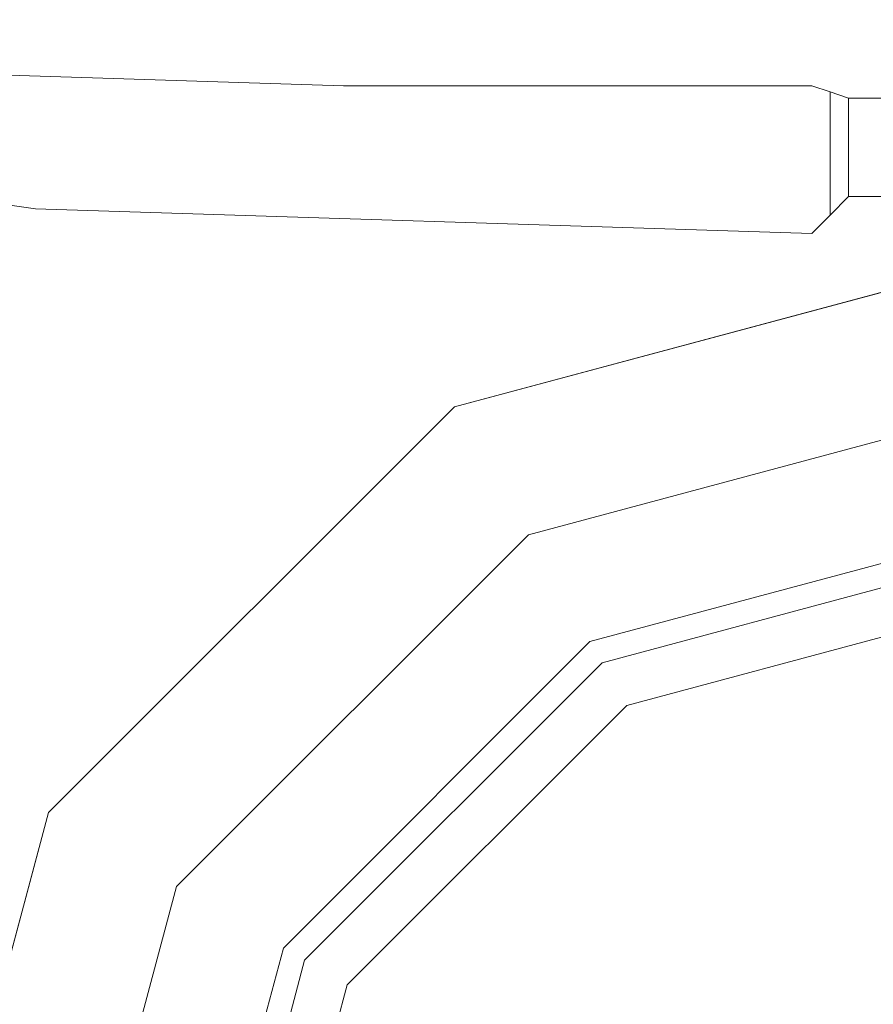
# Model space of a CAD drawing. Units: inches. Extents: x 375 to 1122, y 27 to 1069.
# Tile 144 of 155: x 734.829 to 739.094, y 896.928 to 901.848. Entities that reach past the tile are written whole.
import ezdxf

# ---------------------------------------------------------------- set-up
doc = ezdxf.new("R2010")
doc.units = ezdxf.units.IN
doc.layers.add('A-ANNO-DIMS', color=2, linetype='Continuous', lineweight=18)
doc.layers.add('Furniture', color=30, linetype='Continuous', lineweight=18)
doc.styles.get("Standard").update_dxf_attribs({"font": 'arial.ttf'})
doc.dimstyles.new('ISO-25', dxfattribs={"dimtxt": 12, "dimasz": 2.5, "dimexe": 1.5, "dimexo": 1.5, "dimtad": 1, "dimdec": 1, "dimlunit": 3, "dimtxsty": 'Standard', "dimblk": 'ARCHTICK', "dimcen": 2.5, "dimadec": 0, "dimazin": 0, "dimtfac": 1, "dimtdec": 1, "dimtmove": 0, "dimatfit": 3, "dimfxl": 1.5, "dimfxlon": 1, "dimarcsym": 0})

# ---------------------------------------------------------------- blocks, each defined once
blk = doc.blocks.new('A$C403C54AD')
at = {"linetype": 'ByBlock', "invisible_edges": 5}
for points in [[(0.94168, 1.37069, -0.02349), (0.96015, 1.37069, -0.02349), (0.97623, 1.31066, -0.02349), (0.96024, 1.30143, -0.02349)], [(0.97554, 1.37069, -0.03734), (0.94168, 1.37069, -0.02811), (0.96024, 1.30143, -0.02811), (0.98956, 1.31836, -0.03734)], [(0.96015, 1.37069, -0.02349), (0.97862, 1.37069, -0.02965), (0.99223, 1.3199, -0.02965), (0.97623, 1.31066, -0.02349)], [(0.98477, 1.37069, -0.04658), (0.97554, 1.37069, -0.03734), (0.98956, 1.31836, -0.03734), (0.99756, 1.32297, -0.04658)], [(0.97862, 1.37069, -0.02965), (1.0802, 1.37069, -0.02965), (1.0802, 1.37069, -0.02965), (0.99223, 1.3199, -0.02965)], [(0.99223, 1.3199, -0.02965), (1.0802, 1.37069, -0.02965), (1.0802, 1.37069, -0.02965), (1.02941, 1.28271, -0.02965)], [(1.02941, 1.28271, -0.02965), (1.0802, 1.37069, -0.02965), (1.0802, 1.37069, -0.02965), (1.0802, 1.2691, -0.02965)], [(0.99756, 1.32297, -0.04658), (0.98956, 1.31836, -0.03734), (1.02787, 1.28005, -0.03734), (1.03249, 1.28804, -0.04658)], [(0.97623, 1.31066, -0.02349), (0.99223, 1.3199, -0.02965), (1.02941, 1.28271, -0.02965), (1.02018, 1.26672, -0.02349)], [(0.98956, 1.31836, -0.03734), (0.96024, 1.30143, -0.02811), (1.01094, 1.25072, -0.02811), (1.02787, 1.28005, -0.03734)], [(0.96024, 1.30143, -0.02349), (0.97623, 1.31066, -0.02349), (1.02018, 1.26672, -0.02349), (1.01094, 1.25072, -0.02349)], [(1.03249, 1.28804, -0.04658), (1.02787, 1.28005, -0.03734), (1.0802, 1.26602, -0.03734), (1.0802, 1.27526, -0.04658)], [(1.02018, 1.26672, -0.02349), (1.02941, 1.28271, -0.02965), (1.0802, 1.2691, -0.02965), (1.0802, 1.25063, -0.02349)], [(1.02787, 1.28005, -0.03734), (1.01094, 1.25072, -0.02811), (1.0802, 1.23216, -0.02811), (1.0802, 1.26602, -0.03734)], [(1.01094, 1.25072, -0.02349), (1.02018, 1.26672, -0.02349), (1.0802, 1.25063, -0.02349), (1.0802, 1.23216, -0.02349)]]:
    blk.add_3dface(points, dxfattribs=at)
at = {"linetype": 'ByBlock'}
for points in [[(0.94168, 1.37069, -0.02811), (0.94168, 1.37069, -0.02349), (0.96024, 1.30143, -0.02349), (0.96024, 1.30143, -0.02811)], [(0.96024, 1.30143, -0.02811), (0.96024, 1.30143, -0.02349), (1.01094, 1.25072, -0.02349), (1.01094, 1.25072, -0.02811)], [(1.01094, 1.25072, -0.02811), (1.01094, 1.25072, -0.02349), (1.0802, 1.23216, -0.02349), (1.0802, 1.23216, -0.02811)]]:
    blk.add_3dface(points, dxfattribs=at)
for points in [[(0.92167, 1.35068, -0.03581), (0.93398, 1.35068, -0.03581), (0.93398, 1.35684, -0.03581), (0.92167, 1.35684, -0.03581)], [(0.92167, 1.35068, -0.04504), (0.93398, 1.35068, -0.04504), (0.93398, 1.35684, -0.04504), (0.92167, 1.35684, -0.04504)], [(0.93629, 1.34837, -0.03888), (0.9209, 1.34837, -0.03888), (0.92167, 1.35068, -0.03581), (0.93398, 1.35068, -0.03581)], [(0.93629, 1.34837, -0.04196), (0.9209, 1.34837, -0.04196), (0.92167, 1.35068, -0.04504), (0.93398, 1.35068, -0.04504)]]:
    blk.add_3dface(points)
for points, invisible_edges in [([(0.92167, 1.35684, -0.04504), (0.92167, 1.35684, -0.03581), (0.92167, 1.35068, -0.03581), (0.92167, 1.35068, -0.04504)], 4), ([(0.93398, 1.35068, -0.04504), (0.93398, 1.35068, -0.03581), (0.93398, 1.35684, -0.03581), (0.93398, 1.35684, -0.04504)], 1), ([(0.92167, 1.35068, -0.03581), (0.92167, 1.35068, -0.04504), (0.9209, 1.34837, -0.04196), (0.9209, 1.34837, -0.03888)], 5), ([(0.93629, 1.34837, -0.03888), (0.93629, 1.34837, -0.04196), (0.93398, 1.35068, -0.04504), (0.93398, 1.35068, -0.03581)], 5), ([(0.9386, 1.34606, -0.03965), (0.92013, 1.34606, -0.03965), (0.9209, 1.34837, -0.03888), (0.93629, 1.34837, -0.03888)], 1), ([(0.9386, 1.34606, -0.04119), (0.92013, 1.34606, -0.04119), (0.9209, 1.34837, -0.04196), (0.93629, 1.34837, -0.04196)], 1), ([(0.9209, 1.34837, -0.04196), (0.9209, 1.34837, -0.03888), (0.92013, 1.34606, -0.03965), (0.92013, 1.34606, -0.04119)], 5), ([(0.9386, 1.34606, -0.04119), (0.9386, 1.34606, -0.03965), (0.93629, 1.34837, -0.03888), (0.93629, 1.34837, -0.04196)], 5), ([(0.92013, 1.28757, -0.03965), (0.93552, 1.24909, -0.03965), (0.9386, 1.34606, -0.03965), (0.92013, 1.34606, -0.03965)], 5), ([(0.92013, 1.28757, -0.04119), (0.93552, 1.24909, -0.04119), (0.9386, 1.34606, -0.04119), (0.92013, 1.34606, -0.04119)], 5), ([(0.92013, 1.34606, -0.03965), (0.92013, 1.34606, -0.04119), (0.92013, 1.28757, -0.04119), (0.92013, 1.28757, -0.03965)], 5), ([(0.93552, 1.24909, -0.04119), (0.93552, 1.24909, -0.03965), (0.9386, 1.34606, -0.03965), (0.9386, 1.34606, -0.04119)], 5), ([(0.93398, 1.23832, -0.03965), (0.91859, 1.23832, -0.03965), (0.92013, 1.28757, -0.03965), (0.93552, 1.24909, -0.03965)], 5), ([(0.93398, 1.23832, -0.04119), (0.91859, 1.23832, -0.04119), (0.92013, 1.28757, -0.04119), (0.93552, 1.24909, -0.04119)], 5), ([(0.92013, 1.28757, -0.04119), (0.92013, 1.28757, -0.03965), (0.91859, 1.23832, -0.03965), (0.91859, 1.23832, -0.04119)], 5), ([(0.93398, 1.23832, -0.03965), (0.93398, 1.23832, -0.04119), (0.93552, 1.24909, -0.04119), (0.93552, 1.24909, -0.03965)], 5)]:
    blk.add_3dface(points, dxfattribs=dict(invisible_edges=invisible_edges))
blk = doc.blocks.new('_ArchTick')
at = {"color": 0, "linetype": 'ByBlock', "const_width": 0.15}
blk.add_lwpolyline([(-0.5, -0.5), (0.5, 0.5)], dxfattribs=at)
blk = doc.blocks.new('*D73')
at = {"layer": 'A-ANNO-DIMS', "color": 0, "lineweight": -2, "transparency": 16777216}
for p, q in [((686.7573, 932.4277), (686.7573, 929.4277)), ((770.7573, 932.4277), (770.7573, 929.4277)), ((686.7573, 930.9277), (770.7573, 930.9277)), ((770.7573, 930.9277), (987.6096, 930.9277))]:
    blk.add_line(p, q, dxfattribs=at)
at = {"layer": 'Defpoints', "color": 0, "transparency": 16777216}
for p in [(686.7573, 943.5277), (770.7573, 943.5277), (770.7573, 930.9277)]:
    blk.add_point(p, dxfattribs=at)
at = {"layer": 'A-ANNO-DIMS', "color": 0, "lineweight": -2, "transparency": 16777216, "xscale": 2.5, "yscale": 2.5, "zscale": 2.5, "rotation": 180}
blk.add_blockref('_ArchTick', (686.7573, 930.9277), dxfattribs=at)
at = {"layer": 'A-ANNO-DIMS', "color": 0, "lineweight": -2, "transparency": 16777216, "xscale": 2.5, "yscale": 2.5, "zscale": 2.5}
blk.add_blockref('_ArchTick', (770.7573, 930.9277), dxfattribs=at)
at = {"layer": 'A-ANNO-DIMS', "color": 0, "transparency": 16777216, "insert": (880.4335, 937.7573), "char_height": 12, "attachment_point": 5}
blk.add_mtext('2-PANEL SLIDER 7\'-0" TYP.', dxfattribs=at)
blk = doc.blocks.new('*D88')
at = {"layer": 'A-ANNO-DIMS', "color": 0, "lineweight": -2, "transparency": 16777216}
for p, q in [((731.0073, 1052.5277), (731.0073, 1055.5277)), ((854.0073, 1052.5277), (854.0073, 1055.5277)), ((731.0073, 1054.0277), (854.0073, 1054.0277))]:
    blk.add_line(p, q, dxfattribs=at)
at = {"layer": 'Defpoints', "color": 0, "transparency": 16777216}
for p in [(854.0073, 1054.0277), (731.0073, 502.5277), (854.0073, 502.5277)]:
    blk.add_point(p, dxfattribs=at)
at = {"layer": 'A-ANNO-DIMS', "color": 0, "lineweight": -2, "transparency": 16777216, "xscale": 2.5, "yscale": 2.5, "zscale": 2.5, "rotation": 180}
blk.add_blockref('_ArchTick', (731.0073, 1054.0277), dxfattribs=at)
at = {"layer": 'A-ANNO-DIMS', "color": 0, "lineweight": -2, "transparency": 16777216, "xscale": 2.5, "yscale": 2.5, "zscale": 2.5}
blk.add_blockref('_ArchTick', (854.0073, 1054.0277), dxfattribs=at)
at = {"layer": 'A-ANNO-DIMS', "color": 0, "transparency": 16777216, "insert": (792.5073, 1060.7837), "char_height": 12, "attachment_point": 5}
blk.add_mtext('10\'-3"', dxfattribs=at)
blk = doc.blocks.new('*D91')
at = {"layer": 'A-ANNO-DIMS', "color": 0, "lineweight": -2, "transparency": 16777216}
for p, q in [((728.0073, 1052.5277), (728.0073, 1055.5277)), ((788.0073, 1052.5277), (788.0073, 1055.5277)), ((728.0073, 1054.0277), (788.0073, 1054.0277))]:
    blk.add_line(p, q, dxfattribs=at)
at = {"layer": 'Defpoints', "color": 0, "transparency": 16777216}
for p in [(788.0073, 1054.0277), (728.0073, 774.0277), (788.0073, 774.0277)]:
    blk.add_point(p, dxfattribs=at)
at = {"layer": 'A-ANNO-DIMS', "color": 0, "lineweight": -2, "transparency": 16777216, "xscale": 2.5, "yscale": 2.5, "zscale": 2.5, "rotation": 180}
blk.add_blockref('_ArchTick', (728.0073, 1054.0277), dxfattribs=at)
at = {"layer": 'A-ANNO-DIMS', "color": 0, "lineweight": -2, "transparency": 16777216, "xscale": 2.5, "yscale": 2.5, "zscale": 2.5}
blk.add_blockref('_ArchTick', (788.0073, 1054.0277), dxfattribs=at)
at = {"layer": 'A-ANNO-DIMS', "color": 0, "transparency": 16777216, "insert": (758.0073, 1060.7796), "char_height": 12, "attachment_point": 5}
blk.add_mtext('5\'-0"', dxfattribs=at)

msp = doc.modelspace()

# ---------------------------------------------------------------- block references
at = {"layer": 'Furniture', "xscale": 39.9918517141215, "yscale": 39.9918517141215, "zscale": 39.9918517141215, "rotation": 270}
msp.add_blockref('A$C403C54AD', (684.9549, 938.3156, 0.024), dxfattribs=at)

# ---------------------------------------------------------------- dimensions: what is measured, and where the dimension line sits
at = {"layer": 'A-ANNO-DIMS'}
for base, p1, p2, picture, middle in [((788.0073, 1054.0277), (728.0073, 774.0277), (788.0073, 774.0277), '*D91', (758.0073, 1060.7796)), ((854.0073, 1054.0277), (731.0073, 502.5277), (854.0073, 502.5277), '*D88', (792.5073, 1060.7837))]:
    dim = msp.add_linear_dim(base=base, p1=p1, p2=p2, dimstyle='ISO-25', override={"dimdec": 1, "dimlfac": 1, "dimrnd": 0, "dimzin": 1, "dimdsep": 46, "dimlunit": 4, "dimfrac": 2}, dxfattribs=at)
    dim.commit()
    dim.dimension.update_dxf_attribs({"geometry": picture, "text_midpoint": middle})
dim = msp.add_linear_dim(base=(770.7573, 930.9277), p1=(686.7573, 943.5277), p2=(770.7573, 943.5277), text='2-PANEL SLIDER <> TYP.', dimstyle='ISO-25', override={"dimdec": 1, "dimlfac": 1, "dimrnd": 0, "dimzin": 1, "dimdsep": 46, "dimlunit": 4, "dimfrac": 2}, dxfattribs=at)
dim.commit()
dim.dimension.update_dxf_attribs({"geometry": '*D73', "text_midpoint": (880.4335, 937.7573)})

doc.saveas('drawing.dxf')
